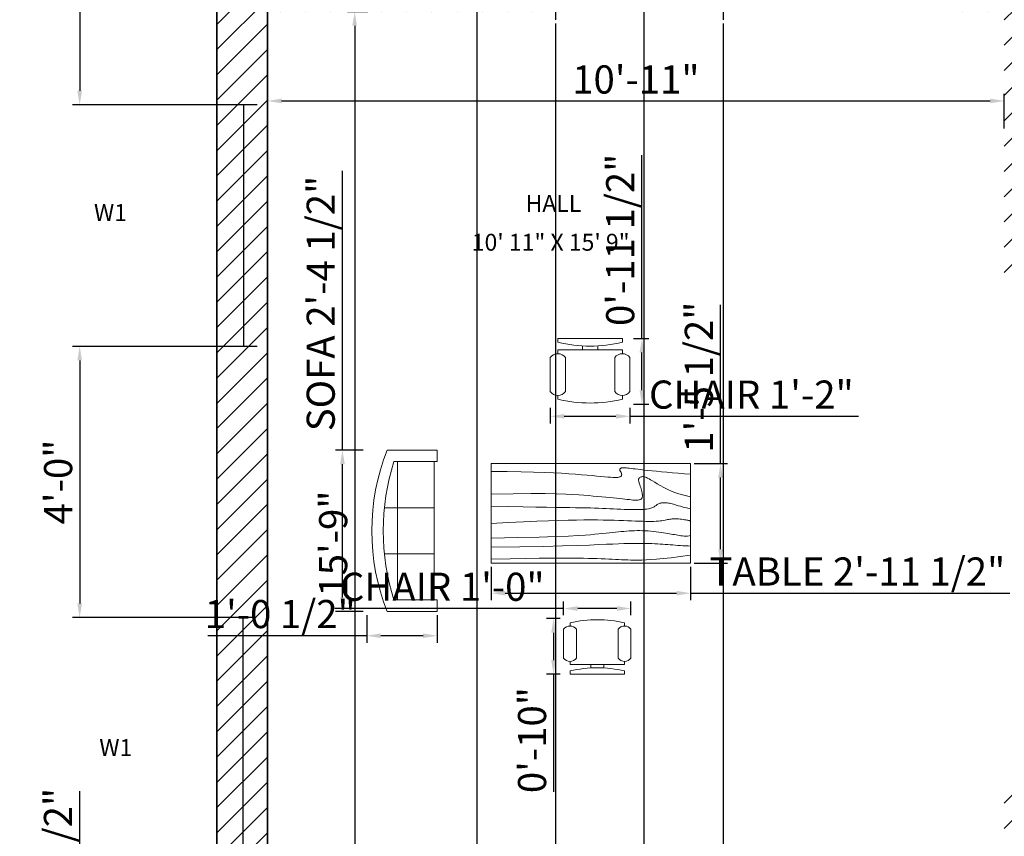
# Model space of a CAD drawing. Units: millimetres. Extents: x 2682 to 3042, y 1647 to 2164.
# Tile 2 of 4: x 2689 to 2864, y 1852 to 1997. Entities that reach past the tile are written whole.
import ezdxf

# ---------------------------------------------------------------- set-up
doc = ezdxf.new("R2010")
doc.units = ezdxf.units.MM
for name, color, linetype, lineweight in [('A-ANNO-TEXT', 170, 'Continuous', 18), ('A-AREA-IDEN', 170, 'Continuous', 18), ('A-WALL-PATT', 3, 'Continuous', 13), ('dimensions', 140, 'Continuous', 18), ('doors', 40, 'Continuous', 25), ('furniture', 220, 'Continuous', 18), ('walls', 70, 'Continuous', 35), ('windows', 50, 'Continuous', 25)]:
    doc.layers.add(name, color=color, linetype=linetype, lineweight=lineweight)
doc.styles.get("Standard").update_dxf_attribs({"font": 'arial.ttf'})
doc.dimstyles.new('ISO-25', dxfattribs={"dimtxt": 5, "dimasz": 2.5, "dimexe": 1.25, "dimexo": 0.625, "dimtad": 1, "dimdec": 0, "dimlunit": 3, "dimtxsty": 'Standard', "dimcen": 2.5, "dimadec": 0, "dimazin": 0, "dimtfac": 1, "dimtdec": 0, "dimtmove": 0, "dimatfit": 3, "dimfxl": 1, "dimarcsym": 0})

# ---------------------------------------------------------------- blocks, each defined once
blk = doc.blocks.new('*U2')
for p, q in [((0, 0), (0, -6)), ((40, 0), (40, -6))]:
    blk.add_line(p, q)
blk.add_lwpolyline([(0, 0), (0, 40), (1.75, 40), (1.75, 0)], close=True)
blk.add_arc((0, 0), 40, 0, 90)
blk = doc.blocks.new('*U4')
for p, q in [((0, 4), (0, 0)), ((36, 4), (36, 0)), ((0, 2), (36, 2))]:
    blk.add_line(p, q)
blk = doc.blocks.new('*D25')
at = {"layer": 'Defpoints', "color": 0, "transparency": 16777216}
for p in [(2751.08, 1998.43), (2748.1, 1809.43), (2751.08, 1809.43)]:
    blk.add_point(p, dxfattribs=at)
at = {"layer": 'dimensions', "color": 0, "lineweight": -2, "transparency": 16777216}
for p, q in [((2750.46, 1998.43), (2746.85, 1998.43)), ((2748.1, 1995.93), (2748.1, 1811.93)), ((2750.46, 1809.43), (2746.85, 1809.43))]:
    blk.add_line(p, q, dxfattribs=at)
at = {"layer": 'dimensions', "color": 0, "transparency": 16777216}
for points in [[(2747.68, 1995.93), (2748.52, 1995.93), (2748.1, 1998.43)], [(2747.68, 1811.93), (2748.52, 1811.93), (2748.1, 1809.43)]]:
    blk.add_solid(points, dxfattribs=at)
at = {"layer": 'dimensions', "color": 0, "transparency": 16777216, "insert": (2744.92, 1903.93), "char_height": 5, "attachment_point": 5, "rotation": 90}
blk.add_mtext('15\'-9"', dxfattribs=at)
blk = doc.blocks.new('*D26')
at = {"layer": 'Defpoints', "color": 0, "transparency": 16777216}
for p in [(2863.59, 1982.58), (2732.59, 1977.09), (2863.59, 1977.09)]:
    blk.add_point(p, dxfattribs=at)
at = {"layer": 'dimensions', "color": 0, "lineweight": -2, "transparency": 16777216}
for p, q in [((2732.59, 1977.71), (2732.59, 1983.83)), ((2863.59, 1977.71), (2863.59, 1983.83)), ((2735.09, 1982.58), (2861.09, 1982.58))]:
    blk.add_line(p, q, dxfattribs=at)
at = {"layer": 'dimensions', "color": 0, "transparency": 16777216}
for points in [[(2735.09, 1982.99), (2735.09, 1982.16), (2732.59, 1982.58)], [(2861.09, 1982.99), (2861.09, 1982.16), (2863.59, 1982.58)]]:
    blk.add_solid(points, dxfattribs=at)
at = {"layer": 'dimensions', "color": 0, "transparency": 16777216, "insert": (2798.09, 1985.75), "char_height": 5, "attachment_point": 5}
blk.add_mtext('10\'-11"', dxfattribs=at)
blk = doc.blocks.new('Sofa - Roundback 7 ft.')
for p, q in [((-12.00002, -32.4421), (-12.00003, -6.5971)), ((11.99997, -32.4421), (11.99998, -6.5971)), ((-36.000027, -34), (-36.000027, -11.4696)), ((-35.999844, -13.3819), (35.9998, -13.3819)), ((35.99998, -34), (35.99998, -11.4696)), ((-36.000027, -32.4421), (35.99998, -32.4421))]:
    blk.add_line(p, q)
for points in [[(-36.000027, -34), (-42.000027, -34), (-42.000027, -8)], [(41.99998, -8), (41.99998, -34), (35.99998, -34)]]:
    blk.add_lwpolyline(points)
for centre, radius, start, end in [((0, -114.25), 114.25, 68.43141, 111.5686), ((-0.00001, -127.1968), 121.1968, 72.72033, 107.2797)]:
    blk.add_arc(centre, radius, start, end)
blk = doc.blocks.new('Table - Rectangular Woodgrain 60 x 30 in.')
for p, q in [((0, 0), (0, -30)), ((60, 0), (0, 0)), ((60, -30), (60, 0)), ((0, -30), (60, -30))]:
    blk.add_line(p, q)
for points in [[(0, -2.4), (4.8155, -2.418), (9.0302, -2.4688), (12.709, -2.5477), (15.9167, -2.65), (18.7181, -2.7711), (21.1781, -2.9063), (23.3616, -3.0508), (25.3333, -3.2), (27.1477, -3.3495), (28.8172, -3.4958), (30.3437, -3.636), (31.7291, -3.7667), (32.9756, -3.8849), (34.0849, -3.9875), (35.059, -4.0714), (35.9, -4.1334), (36.6114, -4.1711), (37.2041, -4.1854), (37.6906, -4.1779), (38.0833, -4.15), (38.3948, -4.1034), (38.6375, -4.0396), (38.8239, -3.9602), (38.9666, -3.8667), (39.0764, -3.7608), (39.1573, -3.6448), (39.2116, -3.521), (39.2416, -3.3917), (39.2498, -3.2593), (39.2385, -3.1261), (39.21, -2.9944), (39.1666, -2.8667), (39.111, -2.7447), (39.0468, -2.6281), (38.978, -2.5163), (38.9083, -2.4083), (38.8418, -2.3035), (38.7823, -2.201), (38.7337, -2.1001), (38.7, -2), (38.6844, -1.9003), (38.6875, -1.8021), (38.7094, -1.707), (38.75, -1.6167), (38.8094, -1.5326), (38.8875, -1.4563), (38.9844, -1.3893), (39.1, -1.3333), (39.2351, -1.2896), (39.3937, -1.2583), (39.5804, -1.2396), (39.8, -1.2333), (40.057, -1.2396), (40.3562, -1.2583), (40.7023, -1.2896), (41.1, -1.3333), (41.5547, -1.3895), (42.0755, -1.4573), (42.6721, -1.5361), (43.3542, -1.625), (44.1316, -1.7233), (45.014, -1.8302), (46.0114, -1.9449), (47.1333, -2.0667), (48.3862, -2.1947), (49.7625, -2.3281), (51.2513, -2.4663), (52.8416, -2.6083), (54.5226, -2.7535), (56.2833, -2.9011), (58.1127, -3.0501), (60, -3.2)], [(0, -9.2), (6.5759, -9.0858), (11.9385, -9.0365), (16.2527, -9.0418), (19.6833, -9.0917), (22.3952, -9.1759), (24.5531, -9.2844), (26.322, -9.4069), (27.8666, -9.5333), (29.3241, -9.6553), (30.7203, -9.7719), (32.0532, -9.8837), (33.3208, -9.9917), (34.5213, -10.0965), (35.6526, -10.199), (36.7128, -10.2999), (37.7, -10.4), (38.6129, -10.4996), (39.4531, -10.5969), (40.223, -10.6895), (40.925, -10.775), (41.5613, -10.8512), (42.1344, -10.9156), (42.6465, -10.966), (43.1, -11), (43.4976, -11.0158), (43.8437, -11.0136), (44.143, -10.9942), (44.4, -10.9583), (44.6195, -10.9069), (44.8062, -10.8406), (44.9648, -10.7603), (45.1, -10.6667), (45.2155, -10.5598), (45.3114, -10.4365), (45.3871, -10.2929), (45.4416, -10.125), (45.4743, -9.929), (45.4844, -9.7011), (45.4709, -9.4371), (45.4333, -9.1333), (45.3716, -8.7883), (45.2896, -8.4104), (45.1919, -8.0107), (45.0833, -7.6), (44.9685, -7.1893), (44.8521, -6.7896), (44.7388, -6.4117), (44.6333, -6.0667), (44.54, -5.7628), (44.4614, -5.4979), (44.4001, -5.2675), (44.3583, -5.0667), (44.3384, -4.8909), (44.3427, -4.7354), (44.3736, -4.5956), (44.4333, -4.4667), (44.5236, -4.3453), (44.6427, -4.2333), (44.7884, -4.1339), (44.9583, -4.05), (45.1501, -3.9849), (45.3614, -3.9417), (45.59, -3.9234), (45.8333, -3.9333), (46.0915, -3.9749), (46.3734, -4.0531), (46.6906, -4.1736), (47.0542, -4.3417), (47.4756, -4.5629), (47.9661, -4.8427), (48.5372, -5.1866), (49.2, -5.6), (49.9676, -6.0844), (50.8594, -6.625), (51.8965, -7.2031), (53.1, -7.8), (54.491, -8.3969), (56.0906, -8.975), (57.9199, -9.5156), (60, -10)], [(0, -12.8), (5.1847, -12.9322), (9.6213, -13.0323), (13.3963, -13.1059), (16.5958, -13.1583), (19.3063, -13.1952), (21.614, -13.2219), (23.6054, -13.2439), (25.3666, -13.2667), (26.9728, -13.2947), (28.4531, -13.3281), (29.8256, -13.3663), (31.1083, -13.4083), (32.3191, -13.4535), (33.476, -13.501), (34.597, -13.5501), (35.7, -13.6), (36.7984, -13.6497), (37.8875, -13.6979), (38.9578, -13.743), (40, -13.7833), (41.0047, -13.8174), (41.9625, -13.8438), (42.864, -13.8607), (43.7, -13.8667), (44.4631, -13.8604), (45.1552, -13.8417), (45.7801, -13.8104), (46.3416, -13.7667), (46.8439, -13.7104), (47.2906, -13.6417), (47.6858, -13.5604), (48.0333, -13.4667), (48.3375, -13.3608), (48.6042, -13.2448), (48.8396, -13.121), (49.05, -12.9917), (49.2417, -12.8593), (49.4208, -12.7261), (49.5937, -12.5944), (49.7667, -12.4667), (49.9452, -12.3451), (50.1323, -12.2313), (50.3303, -12.1268), (50.5416, -12.0333), (50.7686, -11.9524), (51.0135, -11.8854), (51.2788, -11.8341), (51.5666, -11.8), (51.8785, -11.7843), (52.2116, -11.7865), (52.562, -11.8059), (52.926, -11.8417), (53.2998, -11.8931), (53.6795, -11.9594), (54.0614, -12.0397), (54.4416, -12.1333), (54.8223, -12.2401), (55.2293, -12.3625), (55.6942, -12.5037), (56.2489, -12.6667), (56.9251, -12.8547), (57.7545, -13.0708), (58.7689, -13.3182), (60, -13.6)], [(0, -18), (5.124, -17.7273), (9.6609, -17.5057), (13.6705, -17.3303), (17.2125, -17.1958), (20.3467, -17.0973), (23.1328, -17.0297), (25.6307, -16.9878), (27.9, -16.9667), (29.9928, -16.9617), (31.9302, -16.9703), (33.7254, -16.9907), (35.3917, -17.0208), (36.9423, -17.0588), (38.3906, -17.1026), (39.7499, -17.1503), (41.0333, -17.2), (42.2519, -17.2496), (43.4073, -17.2969), (44.4986, -17.3395), (45.525, -17.375), (46.4858, -17.4012), (47.3802, -17.4156), (48.2074, -17.416), (48.9667, -17.4), (49.6583, -17.3662), (50.2872, -17.3167), (50.8595, -17.2547), (51.3812, -17.1833), (51.8584, -17.1057), (52.2971, -17.025), (52.7034, -16.9443), (53.0833, -16.8667), (53.443, -16.7951), (53.789, -16.7313), (54.128, -16.6768), (54.4666, -16.6334), (54.8115, -16.6024), (55.1693, -16.5854), (55.5465, -16.5841), (55.95, -16.6), (56.3828, -16.6337), (56.8346, -16.6823), (57.2915, -16.7418), (57.7396, -16.8084), (58.165, -16.878), (58.5539, -16.9469), (58.8924, -17.0111), (59.1666, -17.0667), (59.3679, -17.1107), (59.5078, -17.1438), (59.6032, -17.1675), (59.6708, -17.1833), (59.7275, -17.193), (59.7901, -17.1979), (59.8753, -17.1998), (60, -17.2)], [(0, -22.4), (8.0098, -22.2501), (14.4094, -22.1011), (19.4168, -21.9535), (23.25, -21.8083), (26.1269, -21.6663), (28.2656, -21.5281), (29.884, -21.3947), (31.2, -21.2667), (32.3967, -21.1448), (33.5172, -21.0292), (34.5697, -20.9198), (35.5625, -20.8167), (36.5037, -20.7198), (37.4015, -20.6292), (38.2642, -20.5448), (39.1, -20.4667), (39.9164, -20.3951), (40.7187, -20.3313), (41.5117, -20.2768), (42.3, -20.2333), (43.0883, -20.2024), (43.8812, -20.1854), (44.6836, -20.1841), (45.5, -20.2), (46.3328, -20.234), (47.1747, -20.2844), (48.0163, -20.3488), (48.8479, -20.425), (49.66, -20.5106), (50.4429, -20.6031), (51.1872, -20.7004), (51.8833, -20.8), (52.5246, -20.8999), (53.1166, -20.9995), (53.6681, -21.0983), (54.1875, -21.1958), (54.6834, -21.2919), (55.1646, -21.3859), (55.6394, -21.4777), (56.1167, -21.5667), (56.6028, -21.6515), (57.0961, -21.7266), (57.5929, -21.7852), (58.0896, -21.8208), (58.5823, -21.8268), (59.0674, -21.7964), (59.5412, -21.723), (60, -21.6)], [(0, -25.2), (8.6355, -25.0504), (15.7026, -24.9031), (21.4049, -24.7606), (25.9458, -24.625), (29.529, -24.4988), (32.3578, -24.3844), (34.6359, -24.284), (36.5667, -24.2), (38.3213, -24.1341), (39.9417, -24.0854), (41.437, -24.0523), (42.8167, -24.0333), (44.0901, -24.0268), (45.2667, -24.0313), (46.3557, -24.0451), (47.3667, -24.0667), (48.309, -24.0947), (49.1928, -24.1287), (50.0284, -24.168), (50.826, -24.2125), (51.5959, -24.2617), (52.3483, -24.3151), (53.0935, -24.3725), (53.8417, -24.4334), (54.6009, -24.497), (55.3699, -24.561), (56.1454, -24.6226), (56.9239, -24.6792), (57.7021, -24.7279), (58.4764, -24.7662), (59.2435, -24.7911), (60, -24.8)], [(0, -28.8), (5.6867, -28.6681), (10.45, -28.5698), (14.407, -28.5012), (17.675, -28.4584), (20.3711, -28.4374), (22.6125, -28.4344), (24.5164, -28.4455), (26.2, -28.4667), (27.762, -28.4947), (29.2276, -28.5281), (30.6033, -28.5663), (31.8958, -28.6084), (33.1118, -28.6535), (34.2578, -28.7011), (35.3405, -28.7501), (36.3666, -28.8), (37.3443, -28.8497), (38.288, -28.8974), (39.2137, -28.9412), (40.1375, -28.9792), (41.0753, -29.0093), (42.0432, -29.0297), (43.0572, -29.0384), (44.1333, -29.0333), (45.2936, -29.0114), (46.5843, -28.9641), (48.0579, -28.8816), (49.7666, -28.7542), (51.7629, -28.5721), (54.0989, -28.3255), (56.8272, -28.0048), (60, -27.6)]]:
    blk.add_lwpolyline(points)
blk = doc.blocks.new('Chair - Desk')
for p, q in [((-8.5, 0), (-8.5, -1)), ((-8.5, 0), (8.5, 0)), ((8.5, 0), (8.5, -1)), ((-2, -3), (-2, -1.9355)), ((2, -1.9576), (2, -3)), ((-10.5, -5), (-10.5, -14)), ((-8.5, -3), (-8.5, -4)), ((-8.5, -3), (8.5, -3)), ((-6.5, -14), (-6.5, -5)), ((6.5, -5), (6.5, -14)), ((8.5, -3), (8.5, -4)), ((10.5, -14), (10.5, -5)), ((-8.5, -15), (-8.5, -16)), ((8.5, -15), (8.5, -16))]:
    blk.add_line(p, q)
for centre, radius, start, end in [((0, 34.625), 36.625, 256.5803, 283.4197), ((-8.5, -6.5), 2.5, 36.8699, 143.1301), ((8.5, -6.5), 2.5, 36.8699, 143.1301), ((-8.5, -12.5), 2.5, 216.8699, 323.1301), ((8.5, -12.5), 2.5, 216.8699, 323.1301), ((0, 19.625), 36.625, 256.5803, 283.4197)]:
    blk.add_arc(centre, radius, start, end)
blk = doc.blocks.new('*D39')
at = {"layer": 'Defpoints', "color": 0, "transparency": 16777216}
for p in [(2782.86, 1928.67), (2797.04, 1928.67), (2797.04, 1926.54)]:
    blk.add_point(p, dxfattribs=at)
at = {"layer": 'dimensions', "color": 0, "lineweight": -2, "transparency": 16777216}
for p, q in [((2782.86, 1928.04), (2782.86, 1925.29)), ((2797.04, 1928.04), (2797.04, 1925.29)), ((2785.36, 1926.54), (2794.54, 1926.54)), ((2797.04, 1926.54), (2837.69, 1926.54))]:
    blk.add_line(p, q, dxfattribs=at)
at = {"layer": 'dimensions', "color": 0, "transparency": 16777216}
for points in [[(2785.36, 1926.96), (2785.36, 1926.12), (2782.86, 1926.54)], [(2794.54, 1926.96), (2794.54, 1926.12), (2797.04, 1926.54)]]:
    blk.add_solid(points, dxfattribs=at)
at = {"layer": 'dimensions', "color": 0, "transparency": 16777216, "insert": (2818.62, 1929.75), "char_height": 5, "attachment_point": 5}
blk.add_mtext('CHAIR 1\'-2"', dxfattribs=at)
blk = doc.blocks.new('*D40')
at = {"layer": 'Defpoints', "color": 0, "transparency": 16777216}
for p in [(2797.04, 1940.37), (2799.16, 1940.37), (2797.04, 1928.67)]:
    blk.add_point(p, dxfattribs=at)
at = {"layer": 'dimensions', "color": 0, "lineweight": -2, "transparency": 16777216}
for p, q in [((2799.16, 1940.37), (2799.16, 1972.94)), ((2797.66, 1940.37), (2800.41, 1940.37)), ((2799.16, 1931.17), (2799.16, 1937.87)), ((2797.66, 1928.67), (2800.41, 1928.67))]:
    blk.add_line(p, q, dxfattribs=at)
at = {"layer": 'dimensions', "color": 0, "transparency": 16777216}
for points in [[(2798.75, 1937.87), (2799.58, 1937.87), (2799.16, 1940.37)], [(2798.75, 1931.17), (2799.58, 1931.17), (2799.16, 1928.67)]]:
    blk.add_solid(points, dxfattribs=at)
at = {"layer": 'dimensions', "color": 0, "transparency": 16777216, "insert": (2795.95, 1957.9), "char_height": 5, "attachment_point": 5, "rotation": 90}
blk.add_mtext('0\'-11 1/2"', dxfattribs=at)
blk = doc.blocks.new('*D41')
at = {"layer": 'Defpoints', "color": 0, "transparency": 16777216}
for p in [(2785.25, 1892.39), (2785.25, 1890.59), (2797.22, 1890.59)]:
    blk.add_point(p, dxfattribs=at)
at = {"layer": 'dimensions', "color": 0, "lineweight": -2, "transparency": 16777216}
for p, q in [((2785.25, 1892.39), (2744.6, 1892.39)), ((2785.25, 1891.22), (2785.25, 1893.64)), ((2794.72, 1892.39), (2787.75, 1892.39)), ((2797.22, 1891.22), (2797.22, 1893.64))]:
    blk.add_line(p, q, dxfattribs=at)
at = {"layer": 'dimensions', "color": 0, "transparency": 16777216}
for points in [[(2787.75, 1892.8), (2787.75, 1891.97), (2785.25, 1892.39)], [(2794.72, 1892.8), (2794.72, 1891.97), (2797.22, 1892.39)]]:
    blk.add_solid(points, dxfattribs=at)
at = {"layer": 'dimensions', "color": 0, "transparency": 16777216, "insert": (2763.67, 1895.6), "char_height": 5, "attachment_point": 5}
blk.add_mtext('CHAIR 1\'-0"', dxfattribs=at)
blk = doc.blocks.new('*D42')
at = {"layer": 'Defpoints', "color": 0, "transparency": 16777216}
for p in [(2785.25, 1890.59), (2783.46, 1880.71), (2785.25, 1880.71)]:
    blk.add_point(p, dxfattribs=at)
at = {"layer": 'dimensions', "color": 0, "lineweight": -2, "transparency": 16777216}
for p, q in [((2784.63, 1890.59), (2782.21, 1890.59)), ((2783.46, 1888.09), (2783.46, 1883.21)), ((2784.63, 1880.71), (2782.21, 1880.71)), ((2783.46, 1880.71), (2783.46, 1859.79))]:
    blk.add_line(p, q, dxfattribs=at)
at = {"layer": 'dimensions', "color": 0, "transparency": 16777216}
for points in [[(2783.04, 1888.09), (2783.87, 1888.09), (2783.46, 1890.59)], [(2783.04, 1883.21), (2783.87, 1883.21), (2783.46, 1880.71)]]:
    blk.add_solid(points, dxfattribs=at)
at = {"layer": 'dimensions', "color": 0, "transparency": 16777216, "insert": (2780.28, 1869), "char_height": 5, "attachment_point": 5, "rotation": 90}
blk.add_mtext('0\'-10"', dxfattribs=at)
blk = doc.blocks.new('*D47')
at = {"layer": 'Defpoints', "color": 0, "transparency": 16777216}
for p in [(2745.93, 1920.53), (2750.23, 1920.53), (2750.23, 1891.84)]:
    blk.add_point(p, dxfattribs=at)
at = {"layer": 'dimensions', "color": 0, "lineweight": -2, "transparency": 16777216}
for p, q in [((2745.93, 1920.53), (2745.93, 1970.15)), ((2749.6, 1920.53), (2744.68, 1920.53)), ((2745.93, 1894.34), (2745.93, 1918.03)), ((2749.6, 1891.84), (2744.68, 1891.84))]:
    blk.add_line(p, q, dxfattribs=at)
at = {"layer": 'dimensions', "color": 0, "transparency": 16777216}
for points in [[(2745.51, 1918.03), (2746.34, 1918.03), (2745.93, 1920.53)], [(2745.51, 1894.34), (2746.34, 1894.34), (2745.93, 1891.84)]]:
    blk.add_solid(points, dxfattribs=at)
at = {"layer": 'dimensions', "color": 0, "transparency": 16777216, "insert": (2742.71, 1946.59), "char_height": 5, "attachment_point": 5, "rotation": 90}
blk.add_mtext('SOFA 2\'-4 1/2"', dxfattribs=at)
blk = doc.blocks.new('*D48')
at = {"layer": 'Defpoints', "color": 0, "transparency": 16777216}
for p in [(2750.23, 1891.84), (2762.75, 1891.84), (2750.23, 1887.54)]:
    blk.add_point(p, dxfattribs=at)
at = {"layer": 'dimensions', "color": 0, "lineweight": -2, "transparency": 16777216}
for p, q in [((2750.23, 1891.22), (2750.23, 1886.29)), ((2762.75, 1891.22), (2762.75, 1886.29)), ((2750.23, 1887.54), (2722.01, 1887.54)), ((2760.25, 1887.54), (2752.73, 1887.54))]:
    blk.add_line(p, q, dxfattribs=at)
at = {"layer": 'dimensions', "color": 0, "transparency": 16777216}
for points in [[(2752.73, 1887.96), (2752.73, 1887.13), (2750.23, 1887.54)], [(2760.25, 1887.96), (2760.25, 1887.13), (2762.75, 1887.54)]]:
    blk.add_solid(points, dxfattribs=at)
at = {"layer": 'dimensions', "color": 0, "transparency": 16777216, "insert": (2734.87, 1890.75), "char_height": 5, "attachment_point": 5}
blk.add_mtext('1\'-0 1/2"', dxfattribs=at)
blk = doc.blocks.new('*D49')
at = {"layer": 'Defpoints', "color": 0, "transparency": 16777216}
for p in [(2772.38, 1900.42), (2807.82, 1900.42), (2807.82, 1895.1)]:
    blk.add_point(p, dxfattribs=at)
at = {"layer": 'dimensions', "color": 0, "lineweight": -2, "transparency": 16777216}
for p, q in [((2772.38, 1899.79), (2772.38, 1893.85)), ((2807.82, 1899.79), (2807.82, 1893.85)), ((2774.88, 1895.1), (2805.32, 1895.1)), ((2807.82, 1895.1), (2864.59, 1895.1))]:
    blk.add_line(p, q, dxfattribs=at)
at = {"layer": 'dimensions', "color": 0, "transparency": 16777216}
for points in [[(2774.88, 1895.52), (2774.88, 1894.69), (2772.38, 1895.1)], [(2805.32, 1895.52), (2805.32, 1894.69), (2807.82, 1895.1)]]:
    blk.add_solid(points, dxfattribs=at)
at = {"layer": 'dimensions', "color": 0, "transparency": 16777216, "insert": (2837.46, 1898.31), "char_height": 5, "attachment_point": 5}
blk.add_mtext('TABLE 2\'-11 1/2"', dxfattribs=at)
blk = doc.blocks.new('*D50')
at = {"layer": 'Defpoints', "color": 0, "transparency": 16777216}
for p in [(2807.82, 1918.14), (2813.14, 1918.14), (2807.82, 1900.42)]:
    blk.add_point(p, dxfattribs=at)
at = {"layer": 'dimensions', "color": 0, "lineweight": -2, "transparency": 16777216}
for p, q in [((2813.14, 1918.14), (2813.14, 1946.36)), ((2808.45, 1918.14), (2814.39, 1918.14)), ((2813.14, 1902.92), (2813.14, 1915.64)), ((2808.45, 1900.42), (2814.39, 1900.42))]:
    blk.add_line(p, q, dxfattribs=at)
at = {"layer": 'dimensions', "color": 0, "transparency": 16777216}
for points in [[(2812.72, 1915.64), (2813.55, 1915.64), (2813.14, 1918.14)], [(2812.72, 1902.92), (2813.55, 1902.92), (2813.14, 1900.42)]]:
    blk.add_solid(points, dxfattribs=at)
at = {"layer": 'dimensions', "color": 0, "transparency": 16777216, "insert": (2809.93, 1933.5), "char_height": 5, "attachment_point": 5, "rotation": 90}
blk.add_mtext('1\'-5 1/2"', dxfattribs=at)
blk = doc.blocks.new('*D52')
at = {"layer": 'Defpoints', "color": 0, "transparency": 16777216}
for p in [(2769.81, 2100.93), (2799.51, 2100.93), (2799.51, 1651.55)]:
    blk.add_point(p, dxfattribs=at)
at = {"layer": 'dimensions', "color": 0, "lineweight": -2, "transparency": 16777216}
for p, q in [((2769.81, 2100.31), (2769.81, 1650.3)), ((2799.51, 2100.31), (2799.51, 1650.3)), ((2772.31, 1651.55), (2797.01, 1651.55))]:
    blk.add_line(p, q, dxfattribs=at)
at = {"layer": 'dimensions', "color": 0, "transparency": 16777216}
for points in [[(2772.31, 1651.97), (2772.31, 1651.13), (2769.81, 1651.55)], [(2797.01, 1651.97), (2797.01, 1651.13), (2799.51, 1651.55)]]:
    blk.add_solid(points, dxfattribs=at)
at = {"layer": 'dimensions', "color": 0, "transparency": 16777216, "insert": (2784.66, 1654.76), "char_height": 5, "attachment_point": 5}
blk.add_mtext('2\'-5 1/2"', dxfattribs=at)
blk = doc.blocks.new('*D53')
at = {"layer": 'Defpoints', "color": 0, "transparency": 16777216}
for p in [(2999.09, 2153.3), (2723.59, 2128.93), (2999.09, 1950.43)]:
    blk.add_point(p, dxfattribs=at)
at = {"layer": 'dimensions', "color": 0, "lineweight": -2, "transparency": 16777216}
for p, q in [((2723.59, 2129.55), (2723.59, 2154.55)), ((2726.09, 2153.3), (2996.59, 2153.3)), ((2999.09, 1951.05), (2999.09, 2154.55))]:
    blk.add_line(p, q, dxfattribs=at)
at = {"layer": 'dimensions', "color": 0, "transparency": 16777216}
for points in [[(2726.09, 2153.72), (2726.09, 2152.88), (2723.59, 2153.3)], [(2996.59, 2153.72), (2996.59, 2152.88), (2999.09, 2153.3)]]:
    blk.add_solid(points, dxfattribs=at)
at = {"layer": 'dimensions', "color": 0, "transparency": 16777216, "insert": (2861.34, 2156.51), "char_height": 5, "attachment_point": 5}
blk.add_mtext('22\'-11 1/2"', dxfattribs=at)
blk = doc.blocks.new('*D59')
at = {"layer": 'Defpoints', "color": 0, "transparency": 16777216}
for p in [(2783.8, 1996.99), (2813.59, 1996.99), (2813.59, 1651.55)]:
    blk.add_point(p, dxfattribs=at)
at = {"layer": 'dimensions', "color": 0, "lineweight": -2, "transparency": 16777216}
for p, q in [((2783.8, 1996.36), (2783.8, 1650.3)), ((2813.59, 1996.36), (2813.59, 1650.3)), ((2786.3, 1651.55), (2811.09, 1651.55))]:
    blk.add_line(p, q, dxfattribs=at)
at = {"layer": 'dimensions', "color": 0, "transparency": 16777216}
for points in [[(2786.3, 1651.97), (2786.3, 1651.13), (2783.8, 1651.55)], [(2811.09, 1651.97), (2811.09, 1651.13), (2813.59, 1651.55)]]:
    blk.add_solid(points, dxfattribs=at)
at = {"layer": 'dimensions', "color": 0, "transparency": 16777216, "insert": (2798.69, 1654.73), "char_height": 5, "attachment_point": 5}
blk.add_mtext('2\'-6"', dxfattribs=at)
blk = doc.blocks.new('*D60')
at = {"layer": 'Defpoints', "color": 0, "transparency": 16777216}
for p in [(2699.21, 1831.73), (2863.18, 1831.73), (2863.18, 1810.31)]:
    blk.add_point(p, dxfattribs=at)
at = {"layer": 'dimensions', "color": 0, "lineweight": -2, "transparency": 16777216}
for p, q in [((2699.21, 1831.73), (2699.21, 1859.95)), ((2862.55, 1831.73), (2697.96, 1831.73)), ((2699.21, 1812.81), (2699.21, 1829.23)), ((2862.55, 1810.31), (2697.96, 1810.31))]:
    blk.add_line(p, q, dxfattribs=at)
at = {"layer": 'dimensions', "color": 0, "transparency": 16777216}
for points in [[(2698.8, 1829.23), (2699.63, 1829.23), (2699.21, 1831.73)], [(2698.8, 1812.81), (2699.63, 1812.81), (2699.21, 1810.31)]]:
    blk.add_solid(points, dxfattribs=at)
at = {"layer": 'dimensions', "color": 0, "transparency": 16777216, "insert": (2696, 1847.09), "char_height": 5, "attachment_point": 5, "rotation": 90}
blk.add_mtext('1\'-9 1/2"', dxfattribs=at)
blk = doc.blocks.new('*D68')
at = {"layer": 'Defpoints', "color": 0, "transparency": 16777216}
for p in [(2728.36, 2029.76), (2699.21, 1981.89), (2728.36, 1981.89)]:
    blk.add_point(p, dxfattribs=at)
at = {"layer": 'dimensions', "color": 0, "lineweight": -2, "transparency": 16777216}
for p, q in [((2727.73, 2029.76), (2697.96, 2029.76)), ((2699.21, 2027.26), (2699.21, 1984.39)), ((2727.73, 1981.89), (2697.96, 1981.89))]:
    blk.add_line(p, q, dxfattribs=at)
at = {"layer": 'dimensions', "color": 0, "transparency": 16777216}
for points in [[(2698.8, 2027.26), (2699.63, 2027.26), (2699.21, 2029.76)], [(2698.8, 1984.39), (2699.63, 1984.39), (2699.21, 1981.89)]]:
    blk.add_solid(points, dxfattribs=at)
at = {"layer": 'dimensions', "color": 0, "transparency": 16777216, "insert": (2696.03, 2005.82), "char_height": 5, "attachment_point": 5, "rotation": 90}
blk.add_mtext('4\'-0"', dxfattribs=at)
blk = doc.blocks.new('*D69')
at = {"layer": 'Defpoints', "color": 0, "transparency": 16777216}
for p in [(2728.36, 1938.97), (2699.21, 1890.78), (2728.2, 1890.78)]:
    blk.add_point(p, dxfattribs=at)
at = {"layer": 'dimensions', "color": 0, "lineweight": -2, "transparency": 16777216}
for p, q in [((2727.73, 1938.97), (2697.96, 1938.97)), ((2699.21, 1936.47), (2699.21, 1893.28)), ((2727.58, 1890.78), (2697.96, 1890.78))]:
    blk.add_line(p, q, dxfattribs=at)
at = {"layer": 'dimensions', "color": 0, "transparency": 16777216}
for points in [[(2698.8, 1936.47), (2699.63, 1936.47), (2699.21, 1938.97)], [(2698.8, 1893.28), (2699.63, 1893.28), (2699.21, 1890.78)]]:
    blk.add_solid(points, dxfattribs=at)
at = {"layer": 'dimensions', "color": 0, "transparency": 16777216, "insert": (2696.03, 1914.87), "char_height": 5, "attachment_point": 5, "rotation": 90}
blk.add_mtext('4\'-0"', dxfattribs=at)

msp = doc.modelspace()

# ---------------------------------------------------------------- hatches: boundary and pattern name
at = {"layer": 'A-WALL-PATT'}
h = msp.add_hatch(dxfattribs=at)
h.set_pattern_fill('ANSI31', color=256)
h.paths.add_polyline_path([(2816.59, 2128.93), (2732.59, 2128.93), (2732.59, 2119.93), (2816.59, 2119.93)])
h.paths.add_polyline_path([(2953.09, 2128.93), (2821.09, 2128.93), (2821.09, 2119.93), (2953.09, 2119.93)])
h.paths.add_polyline_path([(2821.09, 2119.93), (2816.59, 2119.93), (2816.59, 2002.93), (2821.09, 2002.93)])
h.paths.add_polyline_path([(2821.09, 2128.93), (2816.59, 2128.93), (2816.59, 2119.93), (2821.09, 2119.93)])
h.paths.add_polyline_path([(2732.59, 2119.93), (2723.59, 2119.93), (2723.59, 2002.93), (2732.59, 2002.93)])
h.paths.add_polyline_path([(2732.59, 2128.93), (2723.59, 2128.93), (2723.59, 2119.93), (2732.59, 2119.93)])
h.paths.add_polyline_path([(2962.09, 2119.93), (2953.09, 2119.93), (2953.09, 2002.93), (2962.09, 2002.93)])
h.paths.add_polyline_path([(2962.09, 2128.93), (2953.09, 2128.93), (2953.09, 2119.93), (2962.09, 2119.93)])
h.paths.add_polyline_path([(2953.09, 2002.93), (2897.45, 2002.93), (2897.45, 2000.43, -0.023466), (2897.35, 1998.43), (2953.09, 1998.43)])
h.paths.add_polyline_path([(2962.09, 1998.43), (2953.09, 1998.43), (2953.09, 1950.43), (2962.09, 1950.43)])
h.paths.add_polyline_path([(2953.09, 1950.43), (2868.09, 1950.43), (2868.09, 1945.93), (2953.09, 1945.93)])
h.paths.add_polyline_path([(2994.59, 1950.43), (2962.09, 1950.43), (2962.09, 1945.93), (2994.59, 1945.93)])
h.paths.add_polyline_path([(2868.09, 1998.43), (2863.59, 1998.43), (2863.59, 1950.43), (2868.09, 1950.43)])
h.paths.add_polyline_path([(2868.09, 2002.93), (2863.59, 2002.93), (2863.59, 1998.43), (2868.09, 1998.43)])
h.paths.add_polyline_path([(2863.59, 2002.93), (2853.46, 2002.93, -0.011786), (2853.49, 2001.52), (2853.49, 1998.43), (2863.59, 1998.43)])
h.paths.add_polyline_path([(2783.8, 2001.45, -0.012351), (2783.84, 2002.93), (2756.59, 2002.93), (2756.59, 2002.69), (2732.59, 2002.93), (2732.59, 1998.43), (2783.8, 1998.43)])
h.paths.add_polyline_path([(2732.59, 2002.93), (2723.59, 2002.93), (2723.59, 1998.43), (2732.59, 1998.43)])
h.paths.add_polyline_path([(2732.59, 1998.43), (2723.59, 1998.43), (2723.59, 1809.43), (2732.59, 1809.43)])
h.paths.add_polyline_path([(2994.59, 1861.93), (2962.09, 1861.93), (2962.09, 1857.43), (2994.59, 1857.43)])
h.paths.add_polyline_path([(2999.09, 1884.37), (2994.59, 1884.37), (2994.59, 1861.93), (2999.09, 1861.93)])
h.paths.add_polyline_path([(2953.09, 1861.93), (2868.09, 1861.93), (2868.09, 1857.43), (2953.09, 1857.43)])
h.paths.add_polyline_path([(2962.09, 1861.93), (2953.09, 1861.93), (2953.09, 1857.43), (2962.09, 1857.43)])
h.paths.add_polyline_path([(2868.09, 1857.43), (2863.59, 1857.43), (2863.59, 1831.73), (2866.39, 1831.73, -0.019816), (2868.09, 1831.66)])
h.paths.add_polyline_path([(2868.09, 1861.93), (2863.59, 1861.93), (2863.59, 1857.43), (2868.09, 1857.43)])
h.paths.add_polyline_path([(2962.09, 1804.93), (2953.09, 1804.93), (2953.09, 1684.93), (2962.09, 1684.93)])
h.paths.add_polyline_path([(2962.09, 1857.43), (2953.09, 1857.43), (2953.09, 1809.43), (2962.09, 1809.43)])
h.paths.add_polyline_path([(2962.09, 1809.43), (2953.09, 1809.43), (2953.09, 1804.93), (2962.09, 1804.93)])
h.paths.add_polyline_path([(2953.09, 1809.43), (2868.09, 1809.43), (2868.09, 1804.93), (2953.09, 1804.93)])
h.paths.add_polyline_path([(2868.09, 1809.43), (2863.59, 1809.43), (2863.59, 1804.93), (2868.09, 1804.93)])
h.paths.add_polyline_path([(2863.59, 1809.43), (2855.42, 1809.43), (2855.42, 1805.73, -0.006742), (2855.41, 1804.93), (2863.59, 1804.93)])
h.paths.add_polyline_path([(2953.09, 1684.93), (2863.59, 1684.93), (2821.09, 1684.93), (2821.09, 1675.93), (2863.59, 1675.93), (2953.09, 1675.93)])
h.paths.add_polyline_path([(2962.09, 1684.93), (2953.09, 1684.93), (2953.09, 1675.93), (2962.09, 1675.93)])
h.paths.add_polyline_path([(2821.09, 1804.93), (2816.59, 1804.93), (2816.59, 1704.93), (2821.09, 1704.93)])
h.paths.add_polyline_path([(2821.09, 1695.93), (2816.59, 1695.93), (2816.59, 1684.93), (2821.09, 1684.93)])
h.paths.add_polyline_path([(2821.09, 1704.93), (2816.59, 1704.93), (2816.59, 1695.93), (2821.09, 1695.93)])
h.paths.add_polyline_path([(2821.09, 1684.93), (2816.59, 1684.93), (2816.59, 1675.93), (2821.09, 1675.93)])
h.paths.add_polyline_path([(2776.38, 1700.56, -0.030957), (2776.65, 1704.93), (2732.59, 1704.93), (2732.59, 1695.93), (2776.38, 1695.93)])
h.paths.add_polyline_path([(2732.59, 1804.93), (2723.59, 1804.93), (2723.59, 1704.93), (2732.59, 1704.93)])
h.paths.add_polyline_path([(2732.59, 1704.93), (2723.59, 1704.93), (2723.59, 1695.93), (2732.59, 1695.93)])
h.paths.add_polyline_path([(2999.09, 1945.93), (2994.59, 1945.93), (2994.59, 1937.59), (2999.09, 1937.59)])
h.paths.add_polyline_path([(2999.09, 1937.59), (2996.77, 1937.59), (2996.77, 1884.37), (2999.09, 1884.37)])
h.paths.add_polyline_path([(2996.77, 1937.59), (2994.59, 1937.59), (2994.59, 1884.37), (2996.77, 1884.37)])
h.paths.add_polyline_path([(2784.83, 1809.43), (2732.59, 1809.43), (2732.59, 1804.93), (2784.84, 1804.93, -0.006742), (2784.83, 1805.73)])
h.paths.add_polyline_path([(2732.59, 1809.43), (2723.59, 1809.43), (2723.59, 1804.93), (2732.59, 1804.93)])

# ---------------------------------------------------------------- linework, layer by layer
at = {"layer": 'walls'}
for p, q in [((2723.59, 2128.93), (2723.59, 1695.93)), ((2732.59, 2128.93), (2732.59, 1695.93))]:
    msp.add_line(p, q, dxfattribs=at)

# ---------------------------------------------------------------- block references
at = {"layer": 'doors', "xscale": -0.744697270728857, "yscale": 0.744697270728857, "zscale": 0.744697270728857}
msp.add_blockref('*U2', (2813.59, 2001.45), dxfattribs=at)
at = {"layer": 'furniture'}
for name, p, xscale, yscale, zscale in [('Chair - Desk', (2789.95, 1940.37), 0.6750125421142822, 0.6750125421142822, 0.6750125421142822), ('Table - Rectangular Woodgrain 60 x 30 in.', (2772.38, 1918.14), 0.5906701092381653, 0.5906701092381653, 0.5906701092381653)]:
    msp.add_blockref(name, p, dxfattribs=dict(at, xscale=xscale, yscale=yscale, zscale=zscale))
for name, p, xscale, yscale, zscale, rotation in [('Sofa - Roundback 7 ft.', (2751.14, 1906.19), 0.3414396204099792, 0.3414396204099792, 0.3414396204099792, 90), ('Chair - Desk', (2791.23, 1880.71), 0.5697856448786205, 0.5697856448786205, 0.5697856448786205, 180)]:
    msp.add_blockref(name, p, dxfattribs=dict(at, xscale=xscale, yscale=yscale, zscale=zscale, rotation=rotation))
at = {"layer": 'windows', "xscale": 1.192221816707046, "yscale": 1.192221816707046, "zscale": 1.192221816707046, "rotation": 270}
for p in [(2725.97, 1981.89), (2725.82, 1890.78)]:
    msp.add_blockref('*U4', p, dxfattribs=at)

# ---------------------------------------------------------------- texts
at = {"layer": 'A-ANNO-TEXT', "char_height": 3, "attachment_point": 1}
for width, insert in [(11.572, (2701.75, 1964.26)), (20.8903, (2702.7, 1869.18))]:
    msp.add_mtext_dynamic_manual_height_columns('W1', width=width, gutter_width=12.5, heights=[0], dxfattribs=dict(at, insert=insert))
at = {"layer": 'A-AREA-IDEN', "char_height": 3, "attachment_point": 1}
for s, width, insert in [('HALL', 66.4596, (2778.48, 1965.86)), ('10\' 11" X 15\' 9"', 36.6319, (2768.91, 1958.97))]:
    msp.add_mtext_dynamic_manual_height_columns(s, width=width, gutter_width=12.5, heights=[0], dxfattribs=dict(at, insert=insert))

# ---------------------------------------------------------------- dimensions: what is measured, and where the dimension line sits
at = {"layer": 'dimensions'}
for base, p1, p2, override, picture, middle in [((2999.09, 2153.3), (2723.59, 2128.93), (2999.09, 1950.43), {"dimdec": 1, "dimlfac": 1, "dimrnd": 0, "dimzin": 1, "dimdsep": 46, "dimlunit": 4, "dimfrac": 2}, '*D53', (2861.34, 2156.51)), ((2799.51, 1651.55), (2769.81, 2100.93), (2799.51, 2100.93), {"dimdec": 1, "dimlfac": 1, "dimrnd": 0, "dimzin": 1, "dimdsep": 46, "dimlunit": 4, "dimfrac": 2}, '*D52', (2784.66, 1654.76)), ((2813.59, 1651.55), (2783.8, 1996.99), (2813.59, 1996.99), {"dimdec": 1, "dimlfac": 1, "dimrnd": 0, "dimzin": 1, "dimdsep": 46, "dimlunit": 4, "dimfrac": 2}, '*D59', (2798.69, 1654.73)), ((2863.59, 1982.58), (2732.59, 1977.09), (2863.59, 1977.09), {"dimclrd": 0, "dimclre": 0, "dimclrt": 0}, '*D26', (2798.09, 1985.75))]:
    dim = msp.add_linear_dim(base=base, p1=p1, p2=p2, dimstyle='ISO-25', override=override, dxfattribs=at)
    dim.commit()
    dim.dimension.update_dxf_attribs({"geometry": picture, "text_midpoint": middle})
for base, p1, p2, angle, override, picture, middle in [((2699.21, 1981.89), (2728.36, 2029.76), (2728.36, 1981.89), 90, {"dimdec": 1, "dimlfac": 1, "dimrnd": 0, "dimzin": 1, "dimdsep": 46, "dimlunit": 4, "dimfrac": 2}, '*D68', (2696.03, 2005.82)), ((2748.1, 1809.43), (2751.08, 1998.43), (2751.08, 1809.43), 90, {"dimclrd": 0, "dimclre": 0, "dimclrt": 0}, '*D25', (2744.92, 1903.93)), ((2799.16, 1940.37), (2797.04, 1928.67), (2797.04, 1940.37), 90, {"dimdec": 1, "dimlfac": 1, "dimrnd": 0, "dimzin": 1, "dimdsep": 46, "dimlunit": 4, "dimfrac": 2}, '*D40', (2795.95, 1957.9)), ((2813.14, 1918.14), (2807.82, 1900.42), (2807.82, 1918.14), 90, {"dimdec": 1, "dimlfac": 1, "dimrnd": 0, "dimzin": 1, "dimdsep": 46, "dimlunit": 4, "dimfrac": 2}, '*D50', (2809.93, 1933.5)), ((2699.21, 1890.78), (2728.36, 1938.97), (2728.2, 1890.78), 90, {"dimdec": 1, "dimlfac": 1, "dimrnd": 0, "dimzin": 1, "dimdsep": 46, "dimlunit": 4, "dimfrac": 2}, '*D69', (2696.03, 1914.87)), ((2750.23, 1887.54), (2762.75, 1891.84), (2750.23, 1891.84), 180, {"dimdec": 1, "dimlfac": 1, "dimrnd": 0, "dimzin": 1, "dimdsep": 46, "dimlunit": 4, "dimfrac": 2}, '*D48', (2734.87, 1890.75)), ((2783.46, 1880.71), (2785.25, 1890.59), (2785.25, 1880.71), 270, {"dimdec": 1, "dimlfac": 1, "dimrnd": 0, "dimzin": 1, "dimdsep": 46, "dimlunit": 4, "dimfrac": 2}, '*D42', (2780.28, 1869)), ((2699.21, 1831.73), (2863.18, 1810.31), (2863.18, 1831.73), 90, {"dimdec": 1, "dimlfac": 1, "dimrnd": 0, "dimzin": 1, "dimdsep": 46, "dimlunit": 4, "dimfrac": 2}, '*D60', (2696, 1847.09))]:
    dim = msp.add_linear_dim(base=base, p1=p1, p2=p2, angle=angle, dimstyle='ISO-25', override=override, dxfattribs=at)
    dim.commit()
    dim.dimension.update_dxf_attribs({"geometry": picture, "text_midpoint": middle})
for base, p1, p2, angle, text, picture, middle in [((2745.93, 1920.53), (2750.23, 1891.84), (2750.23, 1920.53), 90, 'SOFA <>', '*D47', (2742.71, 1946.59)), ((2785.25, 1892.39), (2797.22, 1890.59), (2785.25, 1890.59), 180, 'CHAIR <>', '*D41', (2763.67, 1895.6))]:
    dim = msp.add_linear_dim(base=base, p1=p1, p2=p2, angle=angle, text=text, dimstyle='ISO-25', override={"dimdec": 1, "dimlfac": 1, "dimrnd": 0, "dimzin": 1, "dimdsep": 46, "dimlunit": 4, "dimfrac": 2}, dxfattribs=at)
    dim.commit()
    dim.dimension.update_dxf_attribs({"geometry": picture, "text_midpoint": middle})
for base, p1, p2, text, picture, middle in [((2797.04, 1926.54), (2782.86, 1928.67), (2797.04, 1928.67), 'CHAIR <>', '*D39', (2818.62, 1929.75)), ((2807.82, 1895.1), (2772.38, 1900.42), (2807.82, 1900.42), 'TABLE <>', '*D49', (2837.46, 1898.31))]:
    dim = msp.add_linear_dim(base=base, p1=p1, p2=p2, text=text, dimstyle='ISO-25', override={"dimdec": 1, "dimlfac": 1, "dimrnd": 0, "dimzin": 1, "dimdsep": 46, "dimlunit": 4, "dimfrac": 2}, dxfattribs=at)
    dim.commit()
    dim.dimension.update_dxf_attribs({"geometry": picture, "text_midpoint": middle})

doc.saveas('drawing.dxf')
